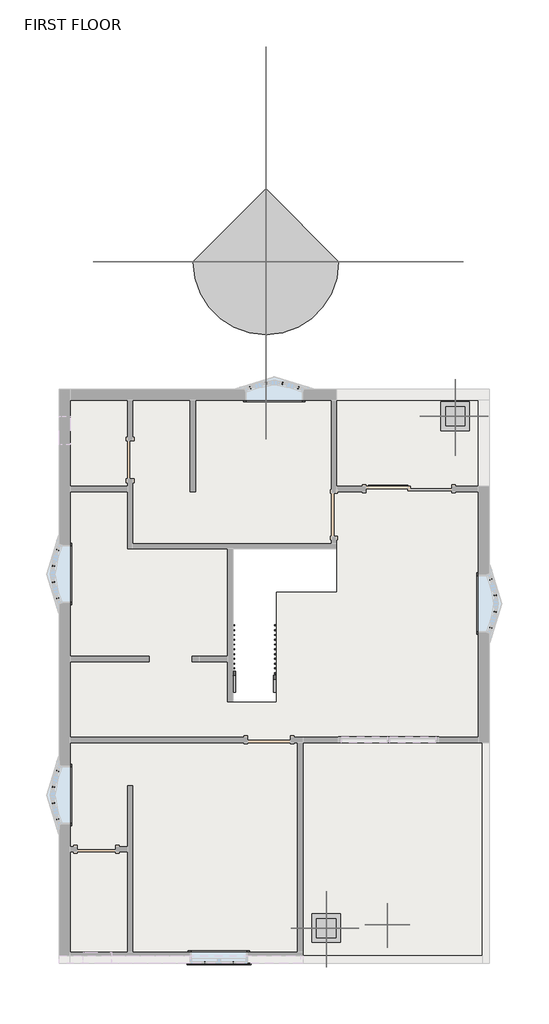
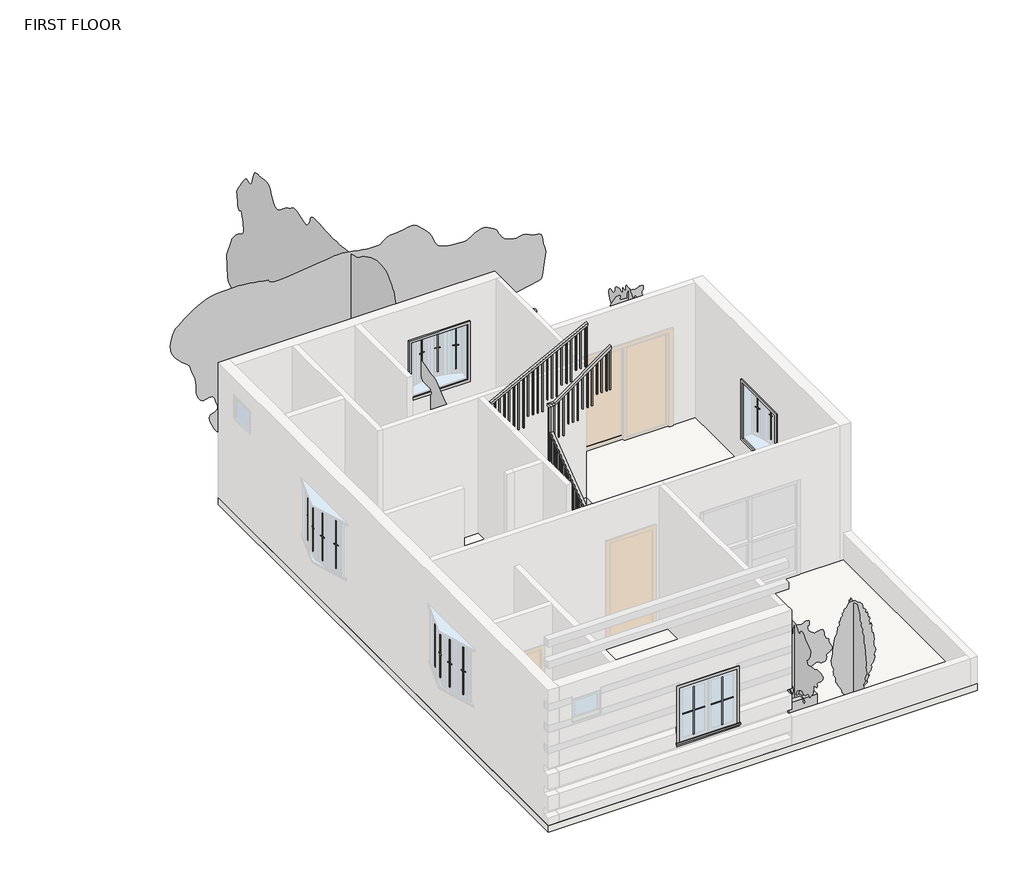
# One storey, part 2 of 2: 24 proxies, 6 geographic elements, 2 railings, 1 slab.
"""IFC4 building model written with IfcOpenShell, lengths in millimetres."""

from ifc_helpers import new_model, si_unit, frame, origin, place, context, project, spatial, polyline, outline, extrude, faceted_brep, transform, mapped, element, save
from components import muntin_pattern_2x2_muntin_pattern_2x2_750a293b, muntin_pattern_2x2_muntin_pattern_2x2_a9af9031, muntin_pattern_2x2_muntin_pattern_2x2_4dfeb3f3, muntin_pattern_2x2_muntin_pattern_2x2_e852a7e4, trim_window_exterior_flat_with_sill_7cfdd449, trim_window_interior_flat_picture_frame_ace0ae79, trim_window_interior_flat_picture_frame_f1e0b15b, planter_2_x2_da431093, rpc_tree_conifer_chinese_juniper_7_1b9786cd, rpc_tree_deciduous_common_apple_20_2_2cf08d23, rpc_tree_deciduous_japanese_cherry_15_720dba75

model = new_model("IFC4")

# Units and contexts
model_context = context("Model", 3, world=origin())
ifc_project = project(units=[si_unit("LENGTHUNIT", "METRE", prefix="MILLI")], contexts=[model_context])

# Site, building, storey
site = spatial("IfcSite", under=ifc_project)
building = spatial("IfcBuilding", under=site)
storey = spatial("IfcBuildingStorey", under=building, Name="FIRST FLOOR", Elevation=3200.4)

# Proxies
placement = place(None, origin())
muntin_pattern_2x2_muntin_pattern_2x2_shape = muntin_pattern_2x2_muntin_pattern_2x2_750a293b(model_context)
element("IfcBuildingElementProxy", 1, Name="Muntin Pattern_2x2 : Muntin Pattern_2x2", ObjectType="Muntin Pattern_2x2 : Muntin Pattern_2x2", at=placement, inside=storey, context=model_context, shape_type="MappedRepresentation", body=[
    mapped(muntin_pattern_2x2_muntin_pattern_2x2_shape, transform((-5861.4497338, -2499.7623237, 4314.7823709), x_axis=(-0.342020143325655, 0.9396926207859135, 0.0), y_axis=(-0.9396926207859135, -0.342020143325655, 0.0), z_axis=(0.0, 0.0, 1.0))),
])
element("IfcBuildingElementProxy", 2, Name="Muntin Pattern_2x2 : Muntin Pattern_2x2", ObjectType="Muntin Pattern_2x2 : Muntin Pattern_2x2", at=placement, inside=storey, context=model_context, shape_type="MappedRepresentation", body=[
    mapped(muntin_pattern_2x2_muntin_pattern_2x2_shape, transform((-5861.4497338, -1476.4532375, 4314.7823709), x_axis=(0.34202014332568176, 0.9396926207859035, 0.0), y_axis=(-0.9396926207859035, 0.34202014332568176, 0.0), z_axis=(0.0, 0.0, 1.0))),
])
element("IfcBuildingElementProxy", 3, Name="Muntin Pattern_2x2 : Muntin Pattern_2x2", ObjectType="Muntin Pattern_2x2 : Muntin Pattern_2x2", at=placement, inside=storey, context=model_context, shape_type="MappedRepresentation", body=[
    mapped(muntin_pattern_2x2_muntin_pattern_2x2_shape, transform((-5952.2870564, -2160.7528206, 4314.7823709), x_axis=(-0.1736481776669109, 0.9848077530122115, 0.0), y_axis=(-0.9848077530122115, -0.1736481776669109, 0.0), z_axis=(0.0, 0.0, 1.0))),
])
element("IfcBuildingElementProxy", 4, Name="Muntin Pattern_2x2 : Muntin Pattern_2x2", ObjectType="Muntin Pattern_2x2 : Muntin Pattern_2x2", at=placement, inside=storey, context=model_context, shape_type="MappedRepresentation", body=[
    mapped(muntin_pattern_2x2_muntin_pattern_2x2_shape, transform((-1766.8960515, 6668.4018239, 4314.7823709), x_axis=(0.9396926207859141, 0.3420201433256534, 0.0), y_axis=(-0.3420201433256534, 0.9396926207859141, 0.0), z_axis=(0.0, 0.0, 1.0))),
])
element("IfcBuildingElementProxy", 5, Name="Muntin Pattern_2x2 : Muntin Pattern_2x2", ObjectType="Muntin Pattern_2x2 : Muntin Pattern_2x2", at=placement, inside=storey, context=model_context, shape_type="MappedRepresentation", body=[
    mapped(muntin_pattern_2x2_muntin_pattern_2x2_shape, transform((-743.5869653, 6668.4018239, 4314.7823709), x_axis=(0.939692620785903, -0.34202014332568337, 0.0), y_axis=(0.34202014332568337, 0.939692620785903, 0.0), z_axis=(0.0, 0.0, 1.0))),
])
element("IfcBuildingElementProxy", 6, Name="Muntin Pattern_2x2 : Muntin Pattern_2x2", ObjectType="Muntin Pattern_2x2 : Muntin Pattern_2x2", at=placement, inside=storey, context=model_context, shape_type="MappedRepresentation", body=[
    mapped(muntin_pattern_2x2_muntin_pattern_2x2_shape, transform((-1427.8865484, 6759.2391465, 4314.7823709), x_axis=(0.9848077530122118, 0.1736481776669092, 0.0), y_axis=(-0.1736481776669092, 0.9848077530122118, 0.0), z_axis=(0.0, 0.0, 1.0))),
])
element("IfcBuildingElementProxy", 7, Name="Muntin Pattern_2x2 : Muntin Pattern_2x2", ObjectType="Muntin Pattern_2x2 : Muntin Pattern_2x2", at=placement, inside=storey, context=model_context, shape_type="MappedRepresentation", body=[
    mapped(muntin_pattern_2x2_muntin_pattern_2x2_shape, transform((-5861.4497338, 2196.9198574, 4314.7823709), x_axis=(-0.342020143325655, 0.9396926207859135, 0.0), y_axis=(-0.9396926207859135, -0.342020143325655, 0.0), z_axis=(0.0, 0.0, 1.0))),
])
element("IfcBuildingElementProxy", 8, Name="Muntin Pattern_2x2 : Muntin Pattern_2x2", ObjectType="Muntin Pattern_2x2 : Muntin Pattern_2x2", at=placement, inside=storey, context=model_context, shape_type="MappedRepresentation", body=[
    mapped(muntin_pattern_2x2_muntin_pattern_2x2_shape, transform((-5861.4497338, 3220.2289436, 4314.7823709), x_axis=(0.34202014332568176, 0.9396926207859035, 0.0), y_axis=(-0.9396926207859035, 0.34202014332568176, 0.0), z_axis=(0.0, 0.0, 1.0))),
])
element("IfcBuildingElementProxy", 9, Name="Muntin Pattern_2x2 : Muntin Pattern_2x2", ObjectType="Muntin Pattern_2x2 : Muntin Pattern_2x2", at=placement, inside=storey, context=model_context, shape_type="MappedRepresentation", body=[
    mapped(muntin_pattern_2x2_muntin_pattern_2x2_shape, transform((-5952.2870564, 2535.9293605, 4314.7823709), x_axis=(-0.1736481776669109, 0.9848077530122115, 0.0), y_axis=(-0.9848077530122115, -0.1736481776669109, 0.0), z_axis=(0.0, 0.0, 1.0))),
])
element("IfcBuildingElementProxy", 10, Name="Muntin Pattern_2x2 : Muntin Pattern_2x2", ObjectType="Muntin Pattern_2x2 : Muntin Pattern_2x2", at=placement, inside=storey, context=model_context, shape_type="MappedRepresentation", body=[
    mapped(muntin_pattern_2x2_muntin_pattern_2x2_shape, transform((3350.9667171, 2592.8981416, 3930.65), x_axis=(0.34202014332565495, -0.9396926207859135, 0.0), y_axis=(0.9396926207859135, 0.34202014332565495, 0.0), z_axis=(0.0, 0.0, 1.0))),
])
element("IfcBuildingElementProxy", 11, Name="Muntin Pattern_2x2 : Muntin Pattern_2x2", ObjectType="Muntin Pattern_2x2 : Muntin Pattern_2x2", at=placement, inside=storey, context=model_context, shape_type="MappedRepresentation", body=[
    mapped(muntin_pattern_2x2_muntin_pattern_2x2_shape, transform((3350.9667171, 1569.5890554, 3930.65), x_axis=(-0.3420201433256818, -0.9396926207859035, 0.0), y_axis=(0.9396926207859035, -0.3420201433256818, 0.0), z_axis=(0.0, 0.0, 1.0))),
])
element("IfcBuildingElementProxy", 12, Name="Muntin Pattern_2x2 : Muntin Pattern_2x2", ObjectType="Muntin Pattern_2x2 : Muntin Pattern_2x2", at=placement, inside=storey, context=model_context, shape_type="MappedRepresentation", body=[
    mapped(muntin_pattern_2x2_muntin_pattern_2x2_shape, transform((3441.8040397, 2253.8886385, 3930.65), x_axis=(0.17364817766691085, -0.9848077530122115, 0.0), y_axis=(0.9848077530122115, 0.17364817766691085, 0.0), z_axis=(0.0, 0.0, 1.0))),
])
muntin_pattern_2x2_muntin_pattern_2x2_2_shape = muntin_pattern_2x2_muntin_pattern_2x2_a9af9031(model_context)
element("IfcBuildingElementProxy", 13, Name="Muntin Pattern_2x2 : Muntin Pattern_2x2", ObjectType="Muntin Pattern_2x2 : Muntin Pattern_2x2", at=placement, inside=storey, context=model_context, shape_type="MappedRepresentation", body=[
    mapped(muntin_pattern_2x2_muntin_pattern_2x2_2_shape, transform((-5952.2870564, -1815.4627406, 4314.7823709), x_axis=(-0.1736481776669139, -0.984807753012211, 0.0), y_axis=(0.984807753012211, -0.1736481776669139, 0.0), z_axis=(0.0, 0.0, 1.0))),
])
element("IfcBuildingElementProxy", 14, Name="Muntin Pattern_2x2 : Muntin Pattern_2x2", ObjectType="Muntin Pattern_2x2 : Muntin Pattern_2x2", at=placement, inside=storey, context=model_context, shape_type="MappedRepresentation", body=[
    mapped(muntin_pattern_2x2_muntin_pattern_2x2_2_shape, transform((-1082.5964684, 6759.2391465, 4314.7823709), x_axis=(-0.9848077530122107, 0.1736481776669156, 0.0), y_axis=(-0.1736481776669156, -0.9848077530122107, 0.0), z_axis=(0.0, 0.0, 1.0))),
])
element("IfcBuildingElementProxy", 15, Name="Muntin Pattern_2x2 : Muntin Pattern_2x2", ObjectType="Muntin Pattern_2x2 : Muntin Pattern_2x2", at=placement, inside=storey, context=model_context, shape_type="MappedRepresentation", body=[
    mapped(muntin_pattern_2x2_muntin_pattern_2x2_2_shape, transform((-5952.2870564, 2881.2194405, 4314.7823709), x_axis=(-0.1736481776669139, -0.984807753012211, 0.0), y_axis=(0.984807753012211, -0.1736481776669139, 0.0), z_axis=(0.0, 0.0, 1.0))),
])
element("IfcBuildingElementProxy", 16, Name="Muntin Pattern_2x2 : Muntin Pattern_2x2", ObjectType="Muntin Pattern_2x2 : Muntin Pattern_2x2", at=placement, inside=storey, context=model_context, shape_type="MappedRepresentation", body=[
    mapped(muntin_pattern_2x2_muntin_pattern_2x2_2_shape, transform((3441.8040397, 1908.5985585, 3930.65), x_axis=(0.17364817766691396, 0.984807753012211, 0.0), y_axis=(-0.984807753012211, 0.17364817766691396, 0.0), z_axis=(0.0, 0.0, 1.0))),
])
muntin_pattern_2x2_muntin_pattern_2x2_3_shape = muntin_pattern_2x2_muntin_pattern_2x2_4dfeb3f3(model_context)
element("IfcBuildingElementProxy", 17, Name="Muntin Pattern_2x2 : Muntin Pattern_2x2", ObjectType="Muntin Pattern_2x2 : Muntin Pattern_2x2", at=placement, inside=storey, context=model_context, shape_type="MappedRepresentation", body=[
    mapped(muntin_pattern_2x2_muntin_pattern_2x2_3_shape, transform((-2130.1595223, -5548.2814015, 4184.65), x_axis=(-1.0, 0.0, 0.0), y_axis=(0.0, -1.0, 0.0), z_axis=(0.0, 0.0, 1.0))),
])
muntin_pattern_2x2_muntin_pattern_2x2_4_shape = muntin_pattern_2x2_muntin_pattern_2x2_e852a7e4(model_context)
element("IfcBuildingElementProxy", 18, Name="Muntin Pattern_2x2 : Muntin Pattern_2x2", ObjectType="Muntin Pattern_2x2 : Muntin Pattern_2x2", at=placement, inside=storey, context=model_context, shape_type="MappedRepresentation", body=[
    mapped(muntin_pattern_2x2_muntin_pattern_2x2_4_shape, transform((-2736.5845223, -5548.2814015, 4184.65), x_axis=(1.0, 0.0, 0.0), y_axis=(0.0, 1.0, 0.0), z_axis=(0.0, 0.0, 1.0))),
])
trim_window_exterior_flat_with_sill_shape = trim_window_exterior_flat_with_sill_7cfdd449(model_context)
element("IfcBuildingElementProxy", 19, Name="Trim-Window-Exterior-Flat : with Sill", ObjectType="Trim-Window-Exterior-Flat : with Sill", at=placement, inside=storey, context=model_context, shape_type="MappedRepresentation", body=[
    mapped(trim_window_exterior_flat_with_sill_shape, transform((-2433.3720223, -5557.8064015, 5334.0), x_axis=(1.0, 0.0, 0.0), y_axis=(0.0, 0.0, 1.0), z_axis=(0.0, -1.0, 0.0))),
])
trim_window_interior_flat_picture_frame_shape = trim_window_interior_flat_picture_frame_ace0ae79(model_context)
element("IfcBuildingElementProxy", 20, Name="Trim-Window-Interior-Flat : Picture Frame", ObjectType="Trim-Window-Interior-Flat : Picture Frame", at=placement, inside=storey, context=model_context, shape_type="MappedRepresentation", body=[
    mapped(trim_window_interior_flat_picture_frame_shape, transform((-5598.6415084, -1988.1077806, 5464.1323709), x_axis=(0.0, 1.0, 0.0), y_axis=(0.0, 0.0, 1.0), z_axis=(1.0, 0.0, 0.0))),
])
element("IfcBuildingElementProxy", 21, Name="Trim-Window-Interior-Flat : Picture Frame", ObjectType="Trim-Window-Interior-Flat : Picture Frame", at=placement, inside=storey, context=model_context, shape_type="MappedRepresentation", body=[
    mapped(trim_window_interior_flat_picture_frame_shape, transform((-1255.2415084, 6405.5935985, 5464.1323709), x_axis=(1.0, 0.0, 0.0), y_axis=(0.0, 0.0, 1.0), z_axis=(0.0, -1.0, 0.0))),
])
element("IfcBuildingElementProxy", 22, Name="Trim-Window-Interior-Flat : Picture Frame", ObjectType="Trim-Window-Interior-Flat : Picture Frame", at=placement, inside=storey, context=model_context, shape_type="MappedRepresentation", body=[
    mapped(trim_window_interior_flat_picture_frame_shape, transform((-5598.6415084, 2708.5744005, 5464.1323709), x_axis=(0.0, 1.0, 0.0), y_axis=(0.0, 0.0, 1.0), z_axis=(1.0, 0.0, 0.0))),
])
element("IfcBuildingElementProxy", 23, Name="Trim-Window-Interior-Flat : Picture Frame", ObjectType="Trim-Window-Interior-Flat : Picture Frame", at=placement, inside=storey, context=model_context, shape_type="MappedRepresentation", body=[
    mapped(trim_window_interior_flat_picture_frame_shape, transform((3088.1584916, 2081.2435985, 5080.0), x_axis=(0.0, -1.0, 0.0), y_axis=(0.0, 0.0, 1.0), z_axis=(-1.0, 0.0, 0.0))),
])
trim_window_interior_flat_picture_frame_2_shape = trim_window_interior_flat_picture_frame_f1e0b15b(model_context)
element("IfcBuildingElementProxy", 24, Name="Trim-Window-Interior-Flat : Picture Frame", ObjectType="Trim-Window-Interior-Flat : Picture Frame", at=placement, inside=storey, context=model_context, shape_type="MappedRepresentation", body=[
    mapped(trim_window_interior_flat_picture_frame_2_shape, transform((-2433.3720223, -5329.2064015, 5334.0), x_axis=(-1.0, 0.0, 0.0), y_axis=(0.0, 0.0, 1.0), z_axis=(0.0, 1.0, 0.0))),
])

# Geographic elements
planter_2_x2_shape = planter_2_x2_da431093(model_context)
element("IfcGeographicElement", 25, ObjectType="Planter : 2'x2'", at=placement, inside=storey, context=model_context, shape_type="MappedRepresentation", body=[
    mapped(planter_2_x2_shape, transform((-150.3415084, -4814.8564015, 3200.4), x_axis=(1.0, 0.0, 0.0), y_axis=(0.0, 1.0, 0.0), z_axis=(0.0, 0.0, 1.0))),
])
element("IfcGeographicElement", 26, ObjectType="Planter : 2'x2'", at=placement, inside=storey, context=model_context, shape_type="MappedRepresentation", body=[
    mapped(planter_2_x2_shape, transform((2592.8584916, 6062.6935985, 3200.4), x_axis=(1.0, 0.0, 0.0), y_axis=(0.0, 1.0, 0.0), z_axis=(0.0, 0.0, 1.0))),
])
rpc_tree_conifer_chinese_juniper_7_shape = rpc_tree_conifer_chinese_juniper_7_1b9786cd(model_context)
element("IfcGeographicElement", 27, ObjectType="RPC Tree - Conifer : Chinese Juniper - 7'", at=placement, inside=storey, context=model_context, shape_type="MappedRepresentation", body=[
    mapped(rpc_tree_conifer_chinese_juniper_7_shape, transform((1144.8618205, -4738.6564015, 3200.4), x_axis=(1.0, 0.0, 0.0), y_axis=(0.0, 1.0, 0.0), z_axis=(0.0, 0.0, 1.0))),
])
rpc_tree_deciduous_common_apple_20_2_shape = rpc_tree_deciduous_common_apple_20_2_2cf08d23(model_context)
element("IfcGeographicElement", 28, ObjectType="RPC Tree - Deciduous : Common Apple - 20' 2", at=placement, inside=storey, context=model_context, shape_type="MappedRepresentation", body=[
    mapped(rpc_tree_deciduous_common_apple_20_2_shape, transform((-1432.9560747, 9347.1078442, -152.4), x_axis=(1.0, 0.0, 0.0), y_axis=(0.0, 1.0, 0.0), z_axis=(0.0, 0.0, 1.0))),
])
rpc_tree_deciduous_japanese_cherry_15_shape = rpc_tree_deciduous_japanese_cherry_15_720dba75(model_context)
element("IfcGeographicElement", 29, ObjectType="RPC Tree - Deciduous : Japanese Cherry - 15'", at=placement, inside=storey, context=model_context, shape_type="MappedRepresentation", body=[
    mapped(rpc_tree_deciduous_japanese_cherry_15_shape, transform((-150.3415084, -4814.8564015, 3200.4), x_axis=(1.0, 0.0, 0.0), y_axis=(0.0, 1.0, 0.0), z_axis=(0.0, 0.0, 1.0))),
])
element("IfcGeographicElement", 30, ObjectType="RPC Tree - Deciduous : Japanese Cherry - 15'", at=placement, inside=storey, context=model_context, shape_type="MappedRepresentation", body=[
    mapped(rpc_tree_deciduous_japanese_cherry_15_shape, transform((2592.8584916, 6062.6935985, 3200.4), x_axis=(1.0, 0.0, 0.0), y_axis=(0.0, 1.0, 0.0), z_axis=(0.0, 0.0, 1.0))),
])

# Railings
element("IfcRailing", 31, ObjectType="Handrail - Rectangular", at=placement, inside=storey, context=model_context, shape_type="SolidModel", body=[
    faceted_brep([(-1267.9415084, 195.2935985, 4191.0), (-1267.9415084, 195.2935985, 4127.5), (-1217.1415084, 195.2935985, 4127.5), (-1217.1415084, 195.2935985, 4191.0), (-1267.9415084, 2252.6935985, 5734.05), (-1267.9415084, 2303.4935985, 5708.65), (-1217.1415084, 2303.4935985, 5708.65), (-1217.1415084, 2252.6935985, 5734.05), (-1267.9415084, 2252.6935985, 6302.7207921), (-1267.9415084, 2303.4935985, 6251.9207921), (-1217.1415084, 2303.4935985, 6251.9207921), (-1217.1415084, 2252.6935985, 6302.7207921), (-1267.9415084, 2379.6935985, 6302.7207921), (-1267.9415084, 2379.6935985, 6251.9207921), (-1217.1415084, 2328.8935985, 6251.9207921), (-1217.1415084, 2328.8935985, 6302.7207921), (-1140.9415084, 2379.6935985, 6302.7207921), (-1124.6881295, 2379.6935985, 6251.9207921), (-1124.6881295, 2328.8935985, 6251.9207921), (-1140.9415084, 2328.8935985, 6302.7207921), (65.5584916, 2379.6935985, 7162.8), (65.5584916, 2328.8935985, 7162.8), (65.5584916, 2328.8935985, 7100.4134329), (65.5584916, 2379.6935985, 7100.4134329)], [[[0, 1, 2, 3]], [[1, 0, 4, 5]], [[2, 1, 5, 6]], [[3, 2, 6, 7]], [[0, 3, 7, 4]], [[5, 4, 8, 9]], [[6, 5, 9, 10]], [[7, 6, 10, 11]], [[4, 7, 11, 8]], [[9, 8, 12, 13]], [[10, 9, 13, 14]], [[11, 10, 14, 15]], [[8, 11, 15, 12]], [[13, 12, 16, 17]], [[14, 13, 17, 18]], [[15, 14, 18, 19]], [[12, 15, 19, 16]], [[20, 21, 22, 23]], [[17, 16, 20, 23]], [[18, 17, 23, 22]], [[19, 18, 22, 21]], [[16, 19, 21, 20]]]),
    extrude(outline(polyline([(7043.8292745, -13.8165084), (7030.2490764, -32.8665084), (6172.2, -32.8665084), (6172.2, -13.8165084), (7043.8292745, -13.8165084)])), frame((0.0, 2344.7685985, 0.0), z_axis=(0.0, 1.0, 0.0), x_axis=(0.0, 0.0, 1.0)), (0.0, 0.0, 1.0), 19.05),
    extrude(outline(polyline([(6971.4015517, -115.4165084), (6957.8213537, -134.4665084), (6172.2, -134.4665084), (6172.2, -115.4165084), (6971.4015517, -115.4165084)])), frame((0.0, 2344.7685985, 0.0), z_axis=(0.0, 1.0, 0.0), x_axis=(0.0, 0.0, 1.0)), (0.0, 0.0, 1.0), 19.05),
    extrude(outline(polyline([(6898.9738289, -217.0165084), (6885.3936309, -236.0665084), (6172.2, -236.0665084), (6172.2, -217.0165084), (6898.9738289, -217.0165084)])), frame((0.0, 2344.7685985, 0.0), z_axis=(0.0, 1.0, 0.0), x_axis=(0.0, 0.0, 1.0)), (0.0, 0.0, 1.0), 19.05),
    extrude(outline(polyline([(6826.5461062, -318.6165084), (6812.9659081, -337.6665084), (5943.6, -337.6665084), (5943.6, -318.6165084), (6826.5461062, -318.6165084)])), frame((0.0, 2344.7685985, 0.0), z_axis=(0.0, 1.0, 0.0), x_axis=(0.0, 0.0, 1.0)), (0.0, 0.0, 1.0), 19.05),
    extrude(outline(polyline([(6754.1183834, -420.2165084), (6740.5381854, -439.2665084), (5943.6, -439.2665084), (5943.6, -420.2165084), (6754.1183834, -420.2165084)])), frame((0.0, 2344.7685985, 0.0), z_axis=(0.0, 1.0, 0.0), x_axis=(0.0, 0.0, 1.0)), (0.0, 0.0, 1.0), 19.05),
    extrude(outline(polyline([(6681.6906606, -521.8165084), (6668.1104626, -540.8665084), (5943.6, -540.8665084), (5943.6, -521.8165084), (6681.6906606, -521.8165084)])), frame((0.0, 2344.7685985, 0.0), z_axis=(0.0, 1.0, 0.0), x_axis=(0.0, 0.0, 1.0)), (0.0, 0.0, 1.0), 19.05),
    extrude(outline(polyline([(6609.2629378, -623.4165084), (6595.6827398, -642.4665084), (5715.0, -642.4665084), (5715.0, -623.4165084), (6609.2629378, -623.4165084)])), frame((0.0, 2344.7685985, 0.0), z_axis=(0.0, 1.0, 0.0), x_axis=(0.0, 0.0, 1.0)), (0.0, 0.0, 1.0), 19.05),
    extrude(outline(polyline([(6536.8352151, -725.0165084), (6523.255017, -744.0665084), (5715.0, -744.0665084), (5715.0, -725.0165084), (6536.8352151, -725.0165084)])), frame((0.0, 2344.7685985, 0.0), z_axis=(0.0, 1.0, 0.0), x_axis=(0.0, 0.0, 1.0)), (0.0, 0.0, 1.0), 19.05),
    extrude(outline(polyline([(6464.4074923, -826.6165084), (6450.8272943, -845.6665084), (5715.0, -845.6665084), (5715.0, -826.6165084), (6464.4074923, -826.6165084)])), frame((0.0, 2344.7685985, 0.0), z_axis=(0.0, 1.0, 0.0), x_axis=(0.0, 0.0, 1.0)), (0.0, 0.0, 1.0), 19.05),
    extrude(outline(polyline([(6391.9797695, -928.2165084), (6378.3995715, -947.2665084), (5486.4, -947.2665084), (5486.4, -928.2165084), (6391.9797695, -928.2165084)])), frame((0.0, 2344.7685985, 0.0), z_axis=(0.0, 1.0, 0.0), x_axis=(0.0, 0.0, 1.0)), (0.0, 0.0, 1.0), 19.05),
    extrude(outline(polyline([(6319.5520467, -1029.8165084), (6305.9718487, -1048.8665084), (5486.4, -1048.8665084), (5486.4, -1029.8165084), (6319.5520467, -1029.8165084)])), frame((0.0, 2344.7685985, 0.0), z_axis=(0.0, 1.0, 0.0), x_axis=(0.0, 0.0, 1.0)), (0.0, 0.0, 1.0), 19.05),
    extrude(outline(polyline([(6247.124324, -1131.4165084), (6233.544126, -1150.4665084), (5486.4, -1150.4665084), (5486.4, -1131.4165084), (6247.124324, -1131.4165084)])), frame((0.0, 2344.7685985, 0.0), z_axis=(0.0, 1.0, 0.0), x_axis=(0.0, 0.0, 1.0)), (0.0, 0.0, 1.0), 19.05),
    extrude(outline(polyline([(-1233.0165084, 2319.3685985), (-1252.0665084, 2319.3685985), (-1252.0665084, 2338.4185985), (-1233.0165084, 2338.4185985), (-1233.0165084, 2319.3685985)])), frame((0.0, 0.0, 5029.2), z_axis=(0.0, 0.0, 1.0), x_axis=(1.0, 0.0, 0.0)), (0.0, 0.0, 1.0), 1222.7207921),
    extrude(outline(polyline([(2217.7685985, 5644.35625), (2236.8185985, 5658.64375), (2236.8185985, 4800.6), (2217.7685985, 4800.6), (2217.7685985, 5644.35625)])), frame((-1252.0665084, 0.0, 0.0), z_axis=(1.0, 0.0, 0.0), x_axis=(0.0, 1.0, 0.0)), (0.0, 0.0, 1.0), 19.05),
    extrude(outline(polyline([(2116.1685985, 5568.15625), (2135.2185985, 5582.44375), (2135.2185985, 4800.6), (2116.1685985, 4800.6), (2116.1685985, 5568.15625)])), frame((-1252.0665084, 0.0, 0.0), z_axis=(1.0, 0.0, 0.0), x_axis=(0.0, 1.0, 0.0)), (0.0, 0.0, 1.0), 19.05),
    extrude(outline(polyline([(2014.5685985, 5491.95625), (2033.6185985, 5506.24375), (2033.6185985, 4800.6), (2014.5685985, 4800.6), (2014.5685985, 5491.95625)])), frame((-1252.0665084, 0.0, 0.0), z_axis=(1.0, 0.0, 0.0), x_axis=(0.0, 1.0, 0.0)), (0.0, 0.0, 1.0), 19.05),
    extrude(outline(polyline([(1912.9685985, 5415.75625), (1932.0185985, 5430.04375), (1932.0185985, 4572.0), (1912.9685985, 4572.0), (1912.9685985, 5415.75625)])), frame((-1252.0665084, 0.0, 0.0), z_axis=(1.0, 0.0, 0.0), x_axis=(0.0, 1.0, 0.0)), (0.0, 0.0, 1.0), 19.05),
    extrude(outline(polyline([(1811.3685985, 5339.55625), (1830.4185985, 5353.84375), (1830.4185985, 4572.0), (1811.3685985, 4572.0), (1811.3685985, 5339.55625)])), frame((-1252.0665084, 0.0, 0.0), z_axis=(1.0, 0.0, 0.0), x_axis=(0.0, 1.0, 0.0)), (0.0, 0.0, 1.0), 19.05),
    extrude(outline(polyline([(1709.7685985, 5263.35625), (1728.8185985, 5277.64375), (1728.8185985, 4572.0), (1709.7685985, 4572.0), (1709.7685985, 5263.35625)])), frame((-1252.0665084, 0.0, 0.0), z_axis=(1.0, 0.0, 0.0), x_axis=(0.0, 1.0, 0.0)), (0.0, 0.0, 1.0), 19.05),
    extrude(outline(polyline([(1608.1685985, 5187.15625), (1627.2185985, 5201.44375), (1627.2185985, 4343.4), (1608.1685985, 4343.4), (1608.1685985, 5187.15625)])), frame((-1252.0665084, 0.0, 0.0), z_axis=(1.0, 0.0, 0.0), x_axis=(0.0, 1.0, 0.0)), (0.0, 0.0, 1.0), 19.05),
    extrude(outline(polyline([(1506.5685985, 5110.95625), (1525.6185985, 5125.24375), (1525.6185985, 4343.4), (1506.5685985, 4343.4), (1506.5685985, 5110.95625)])), frame((-1252.0665084, 0.0, 0.0), z_axis=(1.0, 0.0, 0.0), x_axis=(0.0, 1.0, 0.0)), (0.0, 0.0, 1.0), 19.05),
    extrude(outline(polyline([(1404.9685985, 5034.75625), (1424.0185985, 5049.04375), (1424.0185985, 4343.4), (1404.9685985, 4343.4), (1404.9685985, 5034.75625)])), frame((-1252.0665084, 0.0, 0.0), z_axis=(1.0, 0.0, 0.0), x_axis=(0.0, 1.0, 0.0)), (0.0, 0.0, 1.0), 19.05),
    extrude(outline(polyline([(1303.3685985, 4958.55625), (1322.4185985, 4972.84375), (1322.4185985, 4114.8), (1303.3685985, 4114.8), (1303.3685985, 4958.55625)])), frame((-1252.0665084, 0.0, 0.0), z_axis=(1.0, 0.0, 0.0), x_axis=(0.0, 1.0, 0.0)), (0.0, 0.0, 1.0), 19.05),
    extrude(outline(polyline([(1201.7685985, 4882.35625), (1220.8185985, 4896.64375), (1220.8185985, 4114.8), (1201.7685985, 4114.8), (1201.7685985, 4882.35625)])), frame((-1252.0665084, 0.0, 0.0), z_axis=(1.0, 0.0, 0.0), x_axis=(0.0, 1.0, 0.0)), (0.0, 0.0, 1.0), 19.05),
    extrude(outline(polyline([(1100.1685985, 4806.15625), (1119.2185985, 4820.44375), (1119.2185985, 4114.8), (1100.1685985, 4114.8), (1100.1685985, 4806.15625)])), frame((-1252.0665084, 0.0, 0.0), z_axis=(1.0, 0.0, 0.0), x_axis=(0.0, 1.0, 0.0)), (0.0, 0.0, 1.0), 19.05),
    extrude(outline(polyline([(998.5685985, 4729.95625), (1017.6185985, 4744.24375), (1017.6185985, 3886.2), (998.5685985, 3886.2), (998.5685985, 4729.95625)])), frame((-1252.0665084, 0.0, 0.0), z_axis=(1.0, 0.0, 0.0), x_axis=(0.0, 1.0, 0.0)), (0.0, 0.0, 1.0), 19.05),
    extrude(outline(polyline([(896.9685985, 4653.75625), (916.0185985, 4668.04375), (916.0185985, 3886.2), (896.9685985, 3886.2), (896.9685985, 4653.75625)])), frame((-1252.0665084, 0.0, 0.0), z_axis=(1.0, 0.0, 0.0), x_axis=(0.0, 1.0, 0.0)), (0.0, 0.0, 1.0), 19.05),
    extrude(outline(polyline([(795.3685985, 4577.55625), (814.4185985, 4591.84375), (814.4185985, 3886.2), (795.3685985, 3886.2), (795.3685985, 4577.55625)])), frame((-1252.0665084, 0.0, 0.0), z_axis=(1.0, 0.0, 0.0), x_axis=(0.0, 1.0, 0.0)), (0.0, 0.0, 1.0), 19.05),
    extrude(outline(polyline([(693.7685985, 4501.35625), (712.8185985, 4515.64375), (712.8185985, 3657.6), (693.7685985, 3657.6), (693.7685985, 4501.35625)])), frame((-1252.0665084, 0.0, 0.0), z_axis=(1.0, 0.0, 0.0), x_axis=(0.0, 1.0, 0.0)), (0.0, 0.0, 1.0), 19.05),
    extrude(outline(polyline([(592.1685985, 4425.15625), (611.2185985, 4439.44375), (611.2185985, 3657.6), (592.1685985, 3657.6), (592.1685985, 4425.15625)])), frame((-1252.0665084, 0.0, 0.0), z_axis=(1.0, 0.0, 0.0), x_axis=(0.0, 1.0, 0.0)), (0.0, 0.0, 1.0), 19.05),
    extrude(outline(polyline([(490.5685985, 4348.95625), (509.6185985, 4363.24375), (509.6185985, 3657.6), (490.5685985, 3657.6), (490.5685985, 4348.95625)])), frame((-1252.0665084, 0.0, 0.0), z_axis=(1.0, 0.0, 0.0), x_axis=(0.0, 1.0, 0.0)), (0.0, 0.0, 1.0), 19.05),
    extrude(outline(polyline([(388.9685985, 4272.75625), (408.0185985, 4287.04375), (408.0185985, 3429.0), (388.9685985, 3429.0), (388.9685985, 4272.75625)])), frame((-1252.0665084, 0.0, 0.0), z_axis=(1.0, 0.0, 0.0), x_axis=(0.0, 1.0, 0.0)), (0.0, 0.0, 1.0), 19.05),
    extrude(outline(polyline([(287.3685985, 4196.55625), (306.4185985, 4210.84375), (306.4185985, 3429.0), (287.3685985, 3429.0), (287.3685985, 4196.55625)])), frame((-1252.0665084, 0.0, 0.0), z_axis=(1.0, 0.0, 0.0), x_axis=(0.0, 1.0, 0.0)), (0.0, 0.0, 1.0), 19.05),
    extrude(outline(polyline([(-1233.0165084, 2344.7685985), (-1252.0665084, 2344.7685985), (-1252.0665084, 2363.8185985), (-1233.0165084, 2363.8185985), (-1233.0165084, 2344.7685985)])), frame((0.0, 0.0, 5029.2), z_axis=(0.0, 0.0, 1.0), x_axis=(1.0, 0.0, 0.0)), (0.0, 0.0, 1.0), 1222.7207921),
    extrude(outline(polyline([(7100.4134329, 65.5584916), (7086.8332349, 46.5084916), (6172.2, 46.5084916), (6172.2, 65.5584916), (7100.4134329, 65.5584916)])), frame((0.0, 2344.7685985, 0.0), z_axis=(0.0, 1.0, 0.0), x_axis=(0.0, 0.0, 1.0)), (0.0, 0.0, 1.0), 19.05),
    extrude(outline(polyline([(195.2935985, 4127.5), (214.3435985, 4141.7875), (214.3435985, 3429.0), (195.2935985, 3429.0), (195.2935985, 4127.5)])), frame((-1252.0665084, 0.0, 0.0), z_axis=(1.0, 0.0, 0.0), x_axis=(0.0, 1.0, 0.0)), (0.0, 0.0, 1.0), 19.05),
])
element("IfcRailing", 32, ObjectType="Handrail - Rectangular", at=placement, inside=storey, context=model_context, shape_type="SolidModel", body=[
    faceted_brep([(-2131.5415084, 195.2935985, 4191.0), (-2131.5415084, 195.2935985, 4131.7575287), (-2080.7415084, 195.2935985, 4131.7575287), (-2080.7415084, 195.2935985, 4191.0), (-2131.5415084, 3116.2935985, 5943.6), (-2131.5415084, 3167.0935985, 5914.8375287), (-2080.7415084, 3167.0935985, 5914.8375287), (-2080.7415084, 3116.2935985, 5943.6), (-2131.5415084, 3116.2935985, 6085.8693642), (-2131.5415084, 3167.0935985, 6035.0693642), (-2080.7415084, 3167.0935985, 6035.0693642), (-2080.7415084, 3116.2935985, 6085.8693642), (-2131.5415084, 3243.2935985, 6085.8693642), (-2131.5415084, 3243.2935985, 6035.0693642), (-2080.7415084, 3192.4935985, 6035.0693642), (-2080.7415084, 3192.4935985, 6085.8693642), (-2004.5415084, 3243.2935985, 6085.8693642), (-1992.1179416, 3243.2935985, 6035.0693642), (-1992.1179416, 3192.4935985, 6035.0693642), (-2004.5415084, 3192.4935985, 6085.8693642), (65.5584916, 3243.2935985, 7162.8), (65.5584916, 3192.4935985, 7162.8), (65.5584916, 3192.4935985, 7105.5368728), (65.5584916, 3243.2935985, 7105.5368728)], [[[0, 1, 2, 3]], [[1, 0, 4, 5]], [[2, 1, 5, 6]], [[3, 2, 6, 7]], [[0, 3, 7, 4]], [[5, 4, 8, 9]], [[6, 5, 9, 10]], [[7, 6, 10, 11]], [[4, 7, 11, 8]], [[9, 8, 12, 13]], [[10, 9, 13, 14]], [[11, 10, 14, 15]], [[8, 11, 15, 12]], [[13, 12, 16, 17]], [[14, 13, 17, 18]], [[15, 14, 18, 19]], [[12, 15, 19, 16]], [[20, 21, 22, 23]], [[17, 16, 20, 23]], [[18, 17, 23, 22]], [[19, 18, 22, 21]], [[16, 19, 21, 20]]]),
    extrude(outline(polyline([(7080.7608612, 17.9334916), (6172.2, 17.9334916), (6172.2, 36.9834916), (7090.6712658, 36.9834916), (7080.7608612, 17.9334916)])), frame((0.0, 3208.3685985, 0.0), z_axis=(0.0, 1.0, 0.0), x_axis=(0.0, 0.0, 1.0)), (0.0, 0.0, 1.0), 19.05),
    extrude(outline(polyline([(7027.9053699, -83.6665084), (6172.2, -83.6665084), (6172.2, -64.6165084), (7037.8157745, -64.6165084), (7027.9053699, -83.6665084)])), frame((0.0, 3208.3685985, 0.0), z_axis=(0.0, 1.0, 0.0), x_axis=(0.0, 0.0, 1.0)), (0.0, 0.0, 1.0), 19.05),
    extrude(outline(polyline([(6975.0498785, -185.2665084), (6172.2, -185.2665084), (6172.2, -166.2165084), (6984.9602832, -166.2165084), (6975.0498785, -185.2665084)])), frame((0.0, 3208.3685985, 0.0), z_axis=(0.0, 1.0, 0.0), x_axis=(0.0, 0.0, 1.0)), (0.0, 0.0, 1.0), 19.05),
    extrude(outline(polyline([(6922.1943872, -286.8665084), (5943.6, -286.8665084), (5943.6, -267.8165084), (6932.1047918, -267.8165084), (6922.1943872, -286.8665084)])), frame((0.0, 3208.3685985, 0.0), z_axis=(0.0, 1.0, 0.0), x_axis=(0.0, 0.0, 1.0)), (0.0, 0.0, 1.0), 19.05),
    extrude(outline(polyline([(6869.3388959, -388.4665084), (5943.6, -388.4665084), (5943.6, -369.4165084), (6879.2493005, -369.4165084), (6869.3388959, -388.4665084)])), frame((0.0, 3208.3685985, 0.0), z_axis=(0.0, 1.0, 0.0), x_axis=(0.0, 0.0, 1.0)), (0.0, 0.0, 1.0), 19.05),
    extrude(outline(polyline([(6816.4834046, -490.0665084), (5943.6, -490.0665084), (5943.6, -471.0165084), (6826.3938092, -471.0165084), (6816.4834046, -490.0665084)])), frame((0.0, 3208.3685985, 0.0), z_axis=(0.0, 1.0, 0.0), x_axis=(0.0, 0.0, 1.0)), (0.0, 0.0, 1.0), 19.05),
    extrude(outline(polyline([(6763.6279132, -591.6665084), (5715.0, -591.6665084), (5715.0, -572.6165084), (6773.5383179, -572.6165084), (6763.6279132, -591.6665084)])), frame((0.0, 3208.3685985, 0.0), z_axis=(0.0, 1.0, 0.0), x_axis=(0.0, 0.0, 1.0)), (0.0, 0.0, 1.0), 19.05),
    extrude(outline(polyline([(6710.7724219, -693.2665084), (5715.0, -693.2665084), (5715.0, -674.2165084), (6720.6828265, -674.2165084), (6710.7724219, -693.2665084)])), frame((0.0, 3208.3685985, 0.0), z_axis=(0.0, 1.0, 0.0), x_axis=(0.0, 0.0, 1.0)), (0.0, 0.0, 1.0), 19.05),
    extrude(outline(polyline([(6657.9169306, -794.8665084), (5715.0, -794.8665084), (5715.0, -775.8165084), (6667.8273352, -775.8165084), (6657.9169306, -794.8665084)])), frame((0.0, 3208.3685985, 0.0), z_axis=(0.0, 1.0, 0.0), x_axis=(0.0, 0.0, 1.0)), (0.0, 0.0, 1.0), 19.05),
    extrude(outline(polyline([(6605.0614392, -896.4665084), (5486.4, -896.4665084), (5486.4, -877.4165084), (6614.9718439, -877.4165084), (6605.0614392, -896.4665084)])), frame((0.0, 3208.3685985, 0.0), z_axis=(0.0, 1.0, 0.0), x_axis=(0.0, 0.0, 1.0)), (0.0, 0.0, 1.0), 19.05),
    extrude(outline(polyline([(6552.2059479, -998.0665084), (5486.4, -998.0665084), (5486.4, -979.0165084), (6562.1163525, -979.0165084), (6552.2059479, -998.0665084)])), frame((0.0, 3208.3685985, 0.0), z_axis=(0.0, 1.0, 0.0), x_axis=(0.0, 0.0, 1.0)), (0.0, 0.0, 1.0), 19.05),
    extrude(outline(polyline([(6499.3504566, -1099.6665084), (5486.4, -1099.6665084), (5486.4, -1080.6165084), (6509.2608612, -1080.6165084), (6499.3504566, -1099.6665084)])), frame((0.0, 3208.3685985, 0.0), z_axis=(0.0, 1.0, 0.0), x_axis=(0.0, 0.0, 1.0)), (0.0, 0.0, 1.0), 19.05),
    extrude(outline(polyline([(6446.4949652, -1201.2665084), (5486.4, -1201.2665084), (5486.4, -1182.2165084), (6456.4053699, -1182.2165084), (6446.4949652, -1201.2665084)])), frame((0.0, 3208.3685985, 0.0), z_axis=(0.0, 1.0, 0.0), x_axis=(0.0, 0.0, 1.0)), (0.0, 0.0, 1.0), 19.05),
    extrude(outline(polyline([(6393.6394739, -1302.8665084), (5257.8, -1302.8665084), (5257.8, -1283.8165084), (6403.5498785, -1283.8165084), (6393.6394739, -1302.8665084)])), frame((0.0, 3208.3685985, 0.0), z_axis=(0.0, 1.0, 0.0), x_axis=(0.0, 0.0, 1.0)), (0.0, 0.0, 1.0), 19.05),
    extrude(outline(polyline([(6340.7839826, -1404.4665084), (5257.8, -1404.4665084), (5257.8, -1385.4165084), (6350.6943872, -1385.4165084), (6340.7839826, -1404.4665084)])), frame((0.0, 3208.3685985, 0.0), z_axis=(0.0, 1.0, 0.0), x_axis=(0.0, 0.0, 1.0)), (0.0, 0.0, 1.0), 19.05),
    extrude(outline(polyline([(6287.9284913, -1506.0665084), (5257.8, -1506.0665084), (5257.8, -1487.0165084), (6297.8388959, -1487.0165084), (6287.9284913, -1506.0665084)])), frame((0.0, 3208.3685985, 0.0), z_axis=(0.0, 1.0, 0.0), x_axis=(0.0, 0.0, 1.0)), (0.0, 0.0, 1.0), 19.05),
    extrude(outline(polyline([(6235.0729999, -1607.6665084), (5257.8, -1607.6665084), (5257.8, -1588.6165084), (6244.9834046, -1588.6165084), (6235.0729999, -1607.6665084)])), frame((0.0, 3208.3685985, 0.0), z_axis=(0.0, 1.0, 0.0), x_axis=(0.0, 0.0, 1.0)), (0.0, 0.0, 1.0), 19.05),
    extrude(outline(polyline([(6182.2175086, -1709.2665084), (5257.8, -1709.2665084), (5257.8, -1690.2165084), (6192.1279132, -1690.2165084), (6182.2175086, -1709.2665084)])), frame((0.0, 3208.3685985, 0.0), z_axis=(0.0, 1.0, 0.0), x_axis=(0.0, 0.0, 1.0)), (0.0, 0.0, 1.0), 19.05),
    extrude(outline(polyline([(6129.3620173, -1810.8665084), (5257.8, -1810.8665084), (5257.8, -1791.8165084), (6139.2724219, -1791.8165084), (6129.3620173, -1810.8665084)])), frame((0.0, 3208.3685985, 0.0), z_axis=(0.0, 1.0, 0.0), x_axis=(0.0, 0.0, 1.0)), (0.0, 0.0, 1.0), 19.05),
    extrude(outline(polyline([(6076.5065259, -1912.4665084), (5257.8, -1912.4665084), (5257.8, -1893.4165084), (6086.4169306, -1893.4165084), (6076.5065259, -1912.4665084)])), frame((0.0, 3208.3685985, 0.0), z_axis=(0.0, 1.0, 0.0), x_axis=(0.0, 0.0, 1.0)), (0.0, 0.0, 1.0), 19.05),
    extrude(outline(polyline([(6023.6510346, -2014.0665084), (5257.8, -2014.0665084), (5257.8, -1995.0165084), (6033.5614392, -1995.0165084), (6023.6510346, -2014.0665084)])), frame((0.0, 3208.3685985, 0.0), z_axis=(0.0, 1.0, 0.0), x_axis=(0.0, 0.0, 1.0)), (0.0, 0.0, 1.0), 19.05),
    extrude(outline(polyline([(-2115.6665084, 3132.1685985), (-2115.6665084, 3151.2185985), (-2096.6165084, 3151.2185985), (-2096.6165084, 3132.1685985), (-2115.6665084, 3132.1685985)])), frame((0.0, 0.0, 5029.2), z_axis=(0.0, 0.0, 1.0), x_axis=(1.0, 0.0, 0.0)), (0.0, 0.0, 1.0), 1005.8693642),
    extrude(outline(polyline([(3049.6185985, 5844.3525287), (3049.6185985, 5029.2), (3030.5685985, 5029.2), (3030.5685985, 5832.9225287), (3049.6185985, 5844.3525287)])), frame((-2115.6665084, 0.0, 0.0), z_axis=(1.0, 0.0, 0.0), x_axis=(0.0, 1.0, 0.0)), (0.0, 0.0, 1.0), 19.05),
    extrude(outline(polyline([(2948.0185985, 5783.3925287), (2948.0185985, 5029.2), (2928.9685985, 5029.2), (2928.9685985, 5771.9625287), (2948.0185985, 5783.3925287)])), frame((-2115.6665084, 0.0, 0.0), z_axis=(1.0, 0.0, 0.0), x_axis=(0.0, 1.0, 0.0)), (0.0, 0.0, 1.0), 19.05),
    extrude(outline(polyline([(2846.4185985, 5722.4325287), (2846.4185985, 5029.2), (2827.3685985, 5029.2), (2827.3685985, 5711.0025287), (2846.4185985, 5722.4325287)])), frame((-2115.6665084, 0.0, 0.0), z_axis=(1.0, 0.0, 0.0), x_axis=(0.0, 1.0, 0.0)), (0.0, 0.0, 1.0), 19.05),
    extrude(outline(polyline([(2744.8185985, 5661.4725287), (2744.8185985, 5029.2), (2725.7685985, 5029.2), (2725.7685985, 5650.0425287), (2744.8185985, 5661.4725287)])), frame((-2115.6665084, 0.0, 0.0), z_axis=(1.0, 0.0, 0.0), x_axis=(0.0, 1.0, 0.0)), (0.0, 0.0, 1.0), 19.05),
    extrude(outline(polyline([(2643.2185985, 5600.5125287), (2643.2185985, 5029.2), (2624.1685985, 5029.2), (2624.1685985, 5589.0825287), (2643.2185985, 5600.5125287)])), frame((-2115.6665084, 0.0, 0.0), z_axis=(1.0, 0.0, 0.0), x_axis=(0.0, 1.0, 0.0)), (0.0, 0.0, 1.0), 19.05),
    extrude(outline(polyline([(2541.6185985, 5539.5525287), (2541.6185985, 5029.2), (2522.5685985, 5029.2), (2522.5685985, 5528.1225287), (2541.6185985, 5539.5525287)])), frame((-2115.6665084, 0.0, 0.0), z_axis=(1.0, 0.0, 0.0), x_axis=(0.0, 1.0, 0.0)), (0.0, 0.0, 1.0), 19.05),
    extrude(outline(polyline([(2440.0185985, 5478.5925287), (2440.0185985, 5029.2), (2420.9685985, 5029.2), (2420.9685985, 5467.1625287), (2440.0185985, 5478.5925287)])), frame((-2115.6665084, 0.0, 0.0), z_axis=(1.0, 0.0, 0.0), x_axis=(0.0, 1.0, 0.0)), (0.0, 0.0, 1.0), 19.05),
    extrude(outline(polyline([(2338.4185985, 5417.6325287), (2338.4185985, 5029.2), (2319.3685985, 5029.2), (2319.3685985, 5406.2025287), (2338.4185985, 5417.6325287)])), frame((-2115.6665084, 0.0, 0.0), z_axis=(1.0, 0.0, 0.0), x_axis=(0.0, 1.0, 0.0)), (0.0, 0.0, 1.0), 19.05),
    extrude(outline(polyline([(2236.8185985, 5356.6725287), (2236.8185985, 4800.6), (2217.7685985, 4800.6), (2217.7685985, 5345.2425287), (2236.8185985, 5356.6725287)])), frame((-2115.6665084, 0.0, 0.0), z_axis=(1.0, 0.0, 0.0), x_axis=(0.0, 1.0, 0.0)), (0.0, 0.0, 1.0), 19.05),
    extrude(outline(polyline([(2135.2185985, 5295.7125287), (2135.2185985, 4800.6), (2116.1685985, 4800.6), (2116.1685985, 5284.2825287), (2135.2185985, 5295.7125287)])), frame((-2115.6665084, 0.0, 0.0), z_axis=(1.0, 0.0, 0.0), x_axis=(0.0, 1.0, 0.0)), (0.0, 0.0, 1.0), 19.05),
    extrude(outline(polyline([(2033.6185985, 5234.7525287), (2033.6185985, 4800.6), (2014.5685985, 4800.6), (2014.5685985, 5223.3225287), (2033.6185985, 5234.7525287)])), frame((-2115.6665084, 0.0, 0.0), z_axis=(1.0, 0.0, 0.0), x_axis=(0.0, 1.0, 0.0)), (0.0, 0.0, 1.0), 19.05),
    extrude(outline(polyline([(1932.0185985, 5173.7925287), (1932.0185985, 4572.0), (1912.9685985, 4572.0), (1912.9685985, 5162.3625287), (1932.0185985, 5173.7925287)])), frame((-2115.6665084, 0.0, 0.0), z_axis=(1.0, 0.0, 0.0), x_axis=(0.0, 1.0, 0.0)), (0.0, 0.0, 1.0), 19.05),
    extrude(outline(polyline([(1830.4185985, 5112.8325287), (1830.4185985, 4572.0), (1811.3685985, 4572.0), (1811.3685985, 5101.4025287), (1830.4185985, 5112.8325287)])), frame((-2115.6665084, 0.0, 0.0), z_axis=(1.0, 0.0, 0.0), x_axis=(0.0, 1.0, 0.0)), (0.0, 0.0, 1.0), 19.05),
    extrude(outline(polyline([(1728.8185985, 5051.8725287), (1728.8185985, 4572.0), (1709.7685985, 4572.0), (1709.7685985, 5040.4425287), (1728.8185985, 5051.8725287)])), frame((-2115.6665084, 0.0, 0.0), z_axis=(1.0, 0.0, 0.0), x_axis=(0.0, 1.0, 0.0)), (0.0, 0.0, 1.0), 19.05),
    extrude(outline(polyline([(1627.2185985, 4990.9125287), (1627.2185985, 4343.4), (1608.1685985, 4343.4), (1608.1685985, 4979.4825287), (1627.2185985, 4990.9125287)])), frame((-2115.6665084, 0.0, 0.0), z_axis=(1.0, 0.0, 0.0), x_axis=(0.0, 1.0, 0.0)), (0.0, 0.0, 1.0), 19.05),
    extrude(outline(polyline([(1525.6185985, 4929.9525287), (1525.6185985, 4343.4), (1506.5685985, 4343.4), (1506.5685985, 4918.5225287), (1525.6185985, 4929.9525287)])), frame((-2115.6665084, 0.0, 0.0), z_axis=(1.0, 0.0, 0.0), x_axis=(0.0, 1.0, 0.0)), (0.0, 0.0, 1.0), 19.05),
    extrude(outline(polyline([(1424.0185985, 4868.9925287), (1424.0185985, 4343.4), (1404.9685985, 4343.4), (1404.9685985, 4857.5625287), (1424.0185985, 4868.9925287)])), frame((-2115.6665084, 0.0, 0.0), z_axis=(1.0, 0.0, 0.0), x_axis=(0.0, 1.0, 0.0)), (0.0, 0.0, 1.0), 19.05),
    extrude(outline(polyline([(1322.4185985, 4808.0325287), (1322.4185985, 4114.8), (1303.3685985, 4114.8), (1303.3685985, 4796.6025287), (1322.4185985, 4808.0325287)])), frame((-2115.6665084, 0.0, 0.0), z_axis=(1.0, 0.0, 0.0), x_axis=(0.0, 1.0, 0.0)), (0.0, 0.0, 1.0), 19.05),
    extrude(outline(polyline([(1220.8185985, 4747.0725287), (1220.8185985, 4114.8), (1201.7685985, 4114.8), (1201.7685985, 4735.6425287), (1220.8185985, 4747.0725287)])), frame((-2115.6665084, 0.0, 0.0), z_axis=(1.0, 0.0, 0.0), x_axis=(0.0, 1.0, 0.0)), (0.0, 0.0, 1.0), 19.05),
    extrude(outline(polyline([(1119.2185985, 4686.1125287), (1119.2185985, 4114.8), (1100.1685985, 4114.8), (1100.1685985, 4674.6825287), (1119.2185985, 4686.1125287)])), frame((-2115.6665084, 0.0, 0.0), z_axis=(1.0, 0.0, 0.0), x_axis=(0.0, 1.0, 0.0)), (0.0, 0.0, 1.0), 19.05),
    extrude(outline(polyline([(1017.6185985, 4625.1525287), (1017.6185985, 3886.2), (998.5685985, 3886.2), (998.5685985, 4613.7225287), (1017.6185985, 4625.1525287)])), frame((-2115.6665084, 0.0, 0.0), z_axis=(1.0, 0.0, 0.0), x_axis=(0.0, 1.0, 0.0)), (0.0, 0.0, 1.0), 19.05),
    extrude(outline(polyline([(916.0185985, 4564.1925287), (916.0185985, 3886.2), (896.9685985, 3886.2), (896.9685985, 4552.7625287), (916.0185985, 4564.1925287)])), frame((-2115.6665084, 0.0, 0.0), z_axis=(1.0, 0.0, 0.0), x_axis=(0.0, 1.0, 0.0)), (0.0, 0.0, 1.0), 19.05),
    extrude(outline(polyline([(814.4185985, 4503.2325287), (814.4185985, 3886.2), (795.3685985, 3886.2), (795.3685985, 4491.8025287), (814.4185985, 4503.2325287)])), frame((-2115.6665084, 0.0, 0.0), z_axis=(1.0, 0.0, 0.0), x_axis=(0.0, 1.0, 0.0)), (0.0, 0.0, 1.0), 19.05),
    extrude(outline(polyline([(712.8185985, 4442.2725287), (712.8185985, 3657.6), (693.7685985, 3657.6), (693.7685985, 4430.8425287), (712.8185985, 4442.2725287)])), frame((-2115.6665084, 0.0, 0.0), z_axis=(1.0, 0.0, 0.0), x_axis=(0.0, 1.0, 0.0)), (0.0, 0.0, 1.0), 19.05),
    extrude(outline(polyline([(611.2185985, 4381.3125287), (611.2185985, 3657.6), (592.1685985, 3657.6), (592.1685985, 4369.8825287), (611.2185985, 4381.3125287)])), frame((-2115.6665084, 0.0, 0.0), z_axis=(1.0, 0.0, 0.0), x_axis=(0.0, 1.0, 0.0)), (0.0, 0.0, 1.0), 19.05),
    extrude(outline(polyline([(509.6185985, 4320.3525287), (509.6185985, 3657.6), (490.5685985, 3657.6), (490.5685985, 4308.9225287), (509.6185985, 4320.3525287)])), frame((-2115.6665084, 0.0, 0.0), z_axis=(1.0, 0.0, 0.0), x_axis=(0.0, 1.0, 0.0)), (0.0, 0.0, 1.0), 19.05),
    extrude(outline(polyline([(408.0185985, 4259.3925287), (408.0185985, 3429.0), (388.9685985, 3429.0), (388.9685985, 4247.9625287), (408.0185985, 4259.3925287)])), frame((-2115.6665084, 0.0, 0.0), z_axis=(1.0, 0.0, 0.0), x_axis=(0.0, 1.0, 0.0)), (0.0, 0.0, 1.0), 19.05),
    extrude(outline(polyline([(306.4185985, 4198.4325287), (306.4185985, 3429.0), (287.3685985, 3429.0), (287.3685985, 4187.0025287), (306.4185985, 4198.4325287)])), frame((-2115.6665084, 0.0, 0.0), z_axis=(1.0, 0.0, 0.0), x_axis=(0.0, 1.0, 0.0)), (0.0, 0.0, 1.0), 19.05),
    extrude(outline(polyline([(-2115.6665084, 3208.3685985), (-2115.6665084, 3227.4185985), (-2096.6165084, 3227.4185985), (-2096.6165084, 3208.3685985), (-2115.6665084, 3208.3685985)])), frame((0.0, 0.0, 5029.2), z_axis=(0.0, 0.0, 1.0), x_axis=(1.0, 0.0, 0.0)), (0.0, 0.0, 1.0), 1005.8693642),
    extrude(outline(polyline([(7095.6264681, 46.5084916), (6172.2, 46.5084916), (6172.2, 65.5584916), (7105.5368728, 65.5584916), (7095.6264681, 46.5084916)])), frame((0.0, 3208.3685985, 0.0), z_axis=(0.0, 1.0, 0.0), x_axis=(0.0, 0.0, 1.0)), (0.0, 0.0, 1.0), 19.05),
    extrude(outline(polyline([(214.3435985, 4143.1875287), (214.3435985, 3429.0), (195.2935985, 3429.0), (195.2935985, 4131.7575287), (214.3435985, 4143.1875287)])), frame((-2115.6665084, 0.0, 0.0), z_axis=(1.0, 0.0, 0.0), x_axis=(0.0, 1.0, 0.0)), (0.0, 0.0, 1.0), 19.05),
])

# Slab
element("IfcSlab", 33, ObjectType="6\"", at=placement, inside=storey, context=model_context, shape_type="SweptSolid", body=[
    extrude(outline(polyline([(3316.7584916, 6634.1935985), (3316.7584916, -5557.8064015), (-5827.2415084, -5557.8064015), (-5827.2415084, 6634.1935985), (3316.7584916, 6634.1935985)]), holes=[polyline([(-2131.5415084, 3243.2935985), (-2131.5415084, -9.4533727), (-1217.1415084, -9.4533727), (-1217.1415084, 2328.8935985), (65.5584916, 2328.8935985), (65.5584916, 3243.2935985), (-2131.5415084, 3243.2935985)])]), frame((0.0, 0.0, 3048.0), z_axis=(0.0, 0.0, 1.0), x_axis=(1.0, 0.0, 0.0)), (0.0, 0.0, 1.0), 152.4),
])

save(model, "model.ifc")

# Revit data of these elements
# Type "Muntin Pattern_2x2 : Muntin Pattern_2x2"
#   Width [instance default] = 4' - 0"
#   Thickness = 0' - 0 1/2"
#   Height [instance default] = 4' - 0"
#   Distance = 0' - 0 3/4"
#   Interior Material [instance default] = none
#   Exterior Material [instance default] = none
#   Default Elevation = 0
# Type "Trim-Window-Exterior-Flat : with Sill"
#   Trim Width = 0' - 2 1/4"
#   Trim Thickness_Picture Frame = 0' - 1 1/4"
#   Trim Thickness_with Sill = 0' - 0 3/4"
#   Sill Thickness = 0' - 1 1/4"
#   Opening Width [instance default] = 2' - 0"
#   Opening Height [instance default] = 3' - 0"
#   Default Elevation = 4' - 0"
#   Sill = yes
#   Picture Frame = no
#   Trim Material [instance default] = none
# Type "Trim-Window-Interior-Flat : Picture Frame"
#   Trim Thickness_Picture Frame = 0' - 1 1/4"
#   Trim Width = 0' - 2 1/4"
#   Trim Thickness_with Sill = 0' - 0 3/4"
#   Sill Thickness = 0' - 1 1/4"
#   Opening Width [instance default] = 2' - 0"
#   Opening Height [instance default] = 3' - 0"
#   Default Elevation = 4' - 0"
#   Sill = no
#   Picture Frame = yes
#   Trim Material [instance default] = none
# Type "Planter : 2'x2'"
#   Depth = 2' - 0"
#   Height = 2' - 0"
#   Width = 2' - 0"
#   Material = Concrete, Precast
# Type "RPC Tree - Conifer : Chinese Juniper - 7'"
#   built-in parameter 1005198 = "{2, 15},{39, RPC-16-FUM3-UUQ0-UBF0-N000-ST1L-LVER-AU},{1, 0},{1, 0},{2, 35},{1, 8},{5, Color},{1, 0},{1, 0},{3, 0.8},{3, 0.8},{3, 0.8},{1, 8},{7, BBoxMin},{1, 0},{1, 0},{1, 0},{1, 0},{1, 0},{1, 8},{7, BBoxMax},{1, 0},{1, 0},{1, 0},{1, 0},{1, 0},{2, 11},{9, RPCTypeId},{1, 0},{1, 0},{39, RPC-16-FUM3-UUQ0-UBF0-N000-ST1L-LVER-AU},{1, 6},{14, RPCPlantHeight},{1, 0},{1, 0},{1, 7},{2, 11},{7, keyword},{1, 0},{1, 0},{96, :Geometry:RPC:Chinese Juniper:juniperus chinensis:chinese:juniper:cupressaceae:conifer:evergreen},{2, 11},{8, category},{1, 0},{1, 0},{16, :Trees [General]},{2, 11},{12, LocalizedUID},{1, 0},{1, 0},{15, Chinese Juniper},{2, 14},{6, Height},{1, 0},{1, 0},{1, 7},{1, 2},{16, Cast Reflections},{1, 0},{1, 0},{1, 0},{1, 2},{12, Cast Shadows},{1, 0},{1, 0},{1, 1},{1, 2},{9, Lock View},{1, 0},{1, 0},{1, 0},{1, 4},{5, ViewC},{1, 0},{1, 0},{1, 0},{2, 11},{20, AdvancedUIDefinition},{1, 0},{1, 0},{0, },{2, 11},{10, AssetLibID},{1, 0},{1, 0},{36, 4D3F6E72-3F99-4203-98E9-AF80B3C7A7A4},{2, 11},{10, BaseSchema},{1, 0},{1, 0},{9, RPCSchema},{2, 11},{12, ExchangeGUID},{1, 0},{1, 0},{0, },{1, 2},{6, Hidden},{1, 0},{1, 0},{1, 0},{1, 4},{11, RPCCategory},{1, 0},{1, 0},{1, 0},{2, 11},{8, RPCImage},{1, 0},{1, 0},{0, },{1, 4},{13, SchemaVersion},{1, 0},{1, 0},{1, 4},{2, 11},{12, UIDefinition},{1, 0},{1, 0},{0, },{2, 11},{6, UIName},{1, 0},{1, 0},{39, RPC-16-FUM3-UUQ0-UBF0-N000-ST1L-LVER-AU},{2, 11},{11, VersionGUID},{1, 0},{1, 0},{9, RPCSchema},{2, 11},{9, assettype},{1, 0},{1, 0},{11, RPCGeometry},{2, 11},{11, description},{1, 0},{1, 0},{0, },{2, 11},{9, localname},{1, 0},{1, 0},{3, RPC},{2, 11},{9, localtype},{1, 0},{1, 0},{3, RPC},{1, 4},{8, revision},{1, 0},{1, 0},{1, 1},{2, 11},{9, thumbnail},{1, 0},{1, 0},{0, },{1, 4},{7, version},{1, 0},{1, 0},{1, 1},{1, 2},{20, RPC_Cast Reflections},{1, 0},{1, 0},{1, 1},{1, 2},{16, RPC_Cast Shadows},{1, 0},{1, 0},{1, 1},{1, 2},{13, RPC_Lock View},{1, 0},{1, 0},{1, 0},{1, 4},{9, RPC_ViewC},{1, 0},{1, 0},{1, 0},{21, assetlibrary_base.fbx},{1, 5},"
#   built-in parameter 1005195 = "RPC-16-FUM3-UUQ0-UBF0-N000-ST1L-LVER-AU"
#   Type Comments = "Chinese Juniper"
#   Assembly Code = "G2050500"
#   Height = 7' - 0"
#   Description = (empty or 0)
#   Default Elevation = 0
# Type "RPC Tree - Deciduous : Common Apple - 20' 2"
#   built-in parameter 1005198 = "{2, 15},{39, RPC-16-FXGK-4KXX-PJE5-6000-ST1L-LVER-AU},{1, 0},{1, 0},{2, 35},{1, 8},{5, Color},{1, 0},{1, 0},{3, 0.8},{3, 0.8},{3, 0.8},{1, 8},{7, BBoxMin},{1, 0},{1, 0},{1, 0},{1, 0},{1, 0},{1, 8},{7, BBoxMax},{1, 0},{1, 0},{1, 0},{1, 0},{1, 0},{2, 11},{9, RPCTypeId},{1, 0},{1, 0},{39, RPC-16-FXGK-4KXX-PJE5-6000-ST1L-LVER-AU},{1, 6},{14, RPCPlantHeight},{1, 0},{1, 0},{2, 20},{2, 11},{7, keyword},{1, 0},{1, 0},{168, :Geometry:RPC:Common Apple:Malus sylvestris:occurs in southern Ontario near Lakes Erie and Ontario.  Numerous cultivars planted in orchards; naturalized in many places.},{2, 11},{8, category},{1, 0},{1, 0},{16, :Trees [General]},{2, 11},{12, LocalizedUID},{1, 0},{1, 0},{12, Common Apple},{2, 14},{6, Height},{1, 0},{1, 0},{2, 20},{1, 2},{16, Cast Reflections},{1, 0},{1, 0},{1, 0},{1, 2},{12, Cast Shadows},{1, 0},{1, 0},{1, 1},{1, 2},{9, Lock View},{1, 0},{1, 0},{1, 0},{1, 4},{5, ViewC},{1, 0},{1, 0},{1, 0},{2, 11},{20, AdvancedUIDefinition},{1, 0},{1, 0},{0, },{2, 11},{10, AssetLibID},{1, 0},{1, 0},{36, 4D3F6E72-3F99-4203-98E9-AF80B3C7A7A4},{2, 11},{10, BaseSchema},{1, 0},{1, 0},{9, RPCSchema},{2, 11},{12, ExchangeGUID},{1, 0},{1, 0},{0, },{1, 2},{6, Hidden},{1, 0},{1, 0},{1, 0},{1, 4},{11, RPCCategory},{1, 0},{1, 0},{1, 0},{2, 11},{8, RPCImage},{1, 0},{1, 0},{0, },{1, 4},{13, SchemaVersion},{1, 0},{1, 0},{1, 4},{2, 11},{12, UIDefinition},{1, 0},{1, 0},{0, },{2, 11},{6, UIName},{1, 0},{1, 0},{39, RPC-16-FXGK-4KXX-PJE5-6000-ST1L-LVER-AU},{2, 11},{11, VersionGUID},{1, 0},{1, 0},{9, RPCSchema},{2, 11},{9, assettype},{1, 0},{1, 0},{11, RPCGeometry},{2, 11},{11, description},{1, 0},{1, 0},{0, },{2, 11},{9, localname},{1, 0},{1, 0},{3, RPC},{2, 11},{9, localtype},{1, 0},{1, 0},{3, RPC},{1, 4},{8, revision},{1, 0},{1, 0},{1, 1},{2, 11},{9, thumbnail},{1, 0},{1, 0},{0, },{1, 4},{7, version},{1, 0},{1, 0},{1, 1},{1, 2},{20, RPC_Cast Reflections},{1, 0},{1, 0},{1, 1},{1, 2},{16, RPC_Cast Shadows},{1, 0},{1, 0},{1, 1},{1, 2},{13, RPC_Lock View},{1, 0},{1, 0},{1, 0},{1, 4},{9, RPC_ViewC},{1, 0},{1, 0},{1, 0},{21, assetlibrary_base.fbx},{1, 5},"
#   built-in parameter 1005195 = "RPC-16-FXGK-4KXX-PJE5-6000-ST1L-LVER-AU"
#   Type Comments = "Common Apple"
#   Assembly Code = "G2050500"
#   Height = 20' - 0"
#   Default Elevation = 0
# Type "RPC Tree - Deciduous : Japanese Cherry - 15'"
